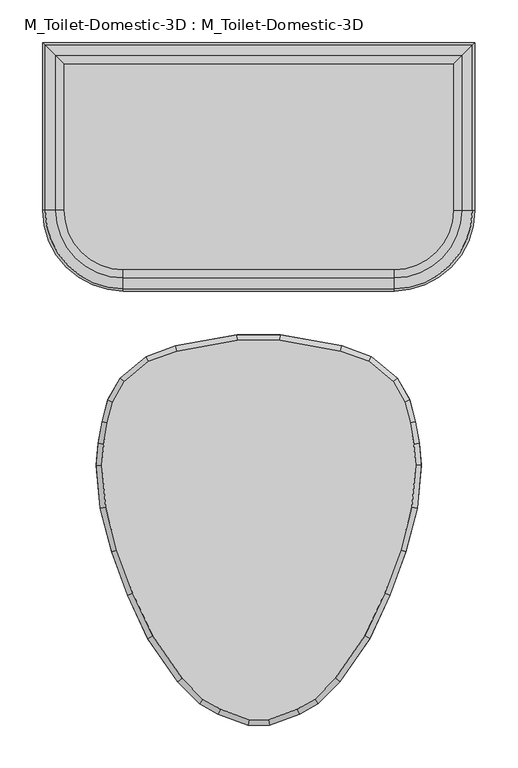
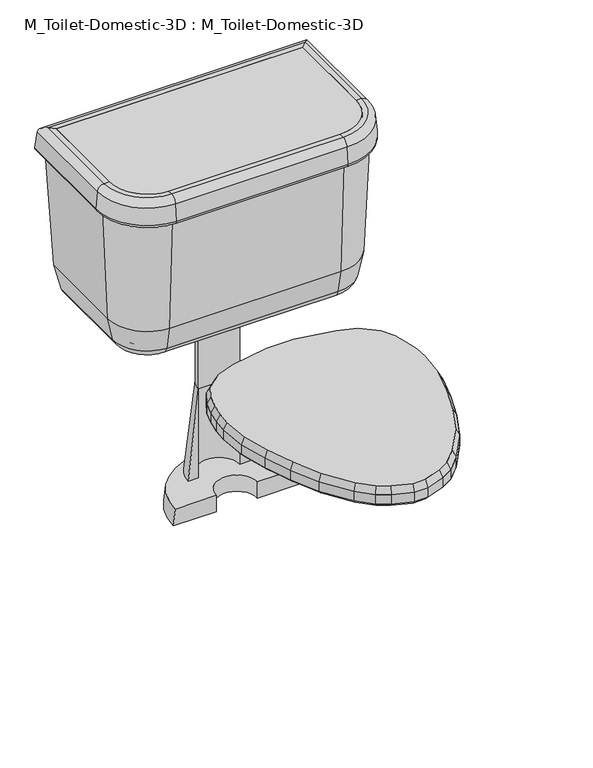
"""IFC4 building model written with IfcOpenShell, lengths in millimetres: flow terminal geometry, M_Toilet-Domestic-3D : M_Toilet-Domestic-3D."""

from ifc_helpers import new_model, si_unit, point, frame, frame_2d, origin, place, context, project, spatial, polyline, circle_curve, ellipse_curve, trimmed, segment, composite_curve, outline, extrude, faceted_brep, source, transform, mapped, element, save
from ifc_brep_helpers import plane_surface, cylinder_surface, revolved_surface, advanced_brep


def m_toilet_domestic_3d_m_toilet_domestic_3d_1a010dbe(model_context):
    return source(origin(), model_context, "Body", "SolidModel", [
        advanced_brep(
        [(177.8, 419.1, 387.2181453), (177.8, 419.1, 374.65), (177.8, 298.45, 374.65), (177.8, 298.45, 387.2181453), (192.8020829, 434.1020829, 387.2181453), (192.8020829, 298.45, 387.2181453), (211.4650931, 452.7650931, 402.4478636), (211.4650931, 298.45, 402.4478636), (218.7732506, 460.0732506, 438.15), (218.7732506, 298.45, 438.15), (228.5868869, 469.8868869, 654.05), (228.5868869, 298.45, 654.05), (228.5868869, 469.8868869, 704.85), (228.5868869, 298.45, 704.85), (237.91817, 479.21817, 704.85), (237.91817, 298.45, 704.85), (250.5698426, 491.8698426, 693.2568779), (250.5698426, 298.45, 693.2568779), (253.3960274, 494.6960274, 660.953439), (253.3960274, 298.45, 660.953439), (247.070191, 488.370191, 654.05), (247.070191, 298.45, 654.05), (241.3, 482.6, 654.05), (241.3, 298.45, 654.05), (231.4863636, 472.7863636, 438.15), (231.4863636, 298.45, 438.15), (222.3416824, 463.6416824, 393.4759963), (222.3416824, 298.45, 393.4759963), (197.8071664, 439.1071664, 374.65), (197.8071664, 298.45, 374.65), (158.75, 279.4, 387.2181453), (158.75, 279.4, 374.65), (158.75, 264.3979171, 387.2181453), (158.75, 245.7349069, 402.4478636), (158.75, 238.4267494, 438.15), (158.75, 228.6131131, 654.05), (158.75, 228.6131131, 704.85), (158.75, 219.28183, 704.85), (158.75, 206.6301574, 693.2568779), (158.75, 203.8039726, 660.953439), (158.75, 210.129809, 654.05), (158.75, 215.9, 654.05), (158.75, 225.7136364, 438.15), (158.75, 234.8583176, 393.4759963), (158.75, 259.3928336, 374.65), (-158.75, 279.4, 374.65), (-158.75, 279.4, 387.2181453), (-158.75, 264.3979171, 387.2181453), (-158.75, 245.7349069, 402.4478636), (-158.75, 238.4267494, 438.15), (-158.75, 228.6131131, 654.05), (-158.75, 228.6131131, 704.85), (-158.75, 219.28183, 704.85), (-158.75, 206.6301574, 693.2568779), (-158.75, 203.8039726, 660.953439), (-158.75, 210.129809, 654.05), (-158.75, 215.9, 654.05), (-158.75, 225.7136364, 438.15), (-158.75, 234.8583176, 393.4759963), (-158.75, 259.3928336, 374.65), (-177.8, 298.45, 387.2181453), (-177.8, 298.45, 374.65), (-192.8020829, 298.45, 387.2181453), (-211.4650931, 298.45, 402.4478636), (-218.7732506, 298.45, 438.15), (-228.5868869, 298.45, 654.05), (-228.5868869, 298.45, 704.85), (-237.91817, 298.45, 704.85), (-250.5698426, 298.45, 693.2568779), (-253.3960274, 298.45, 660.953439), (-247.070191, 298.45, 654.05), (-241.3, 298.45, 654.05), (-231.4863636, 298.45, 438.15), (-222.3416824, 298.45, 393.4759963), (-197.8071664, 298.45, 374.65), (-177.8, 419.1, 374.65), (-177.8, 419.1, 387.2181453), (-192.8020829, 434.1020829, 387.2181453), (-211.4650931, 452.7650931, 402.4478636), (-218.7732506, 460.0732506, 438.15), (-228.5868869, 469.8868869, 654.05), (-228.5868869, 469.8868869, 704.85), (-237.91817, 479.21817, 704.85), (-250.5698426, 491.8698426, 693.2568779), (-253.3960274, 494.6960274, 660.953439), (-247.070191, 488.370191, 654.05), (-241.3, 482.6, 654.05), (-231.4863636, 472.7863636, 438.15), (-222.3416824, 463.6416824, 393.4759963), (-197.8071664, 439.1071664, 374.65)],
        [
            (0, 1),
            (1, 2),
            (2, 3),
            (3, 0),
            (4, 0),
            (3, 5),
            (5, 4),
            (6, 4, ellipse_curve(frame((192.8020829, 434.1020829, 406.2681453), z_axis=(-0.7071067811865451, 0.7071067811865498, 0.0), x_axis=(-0.7071067811865497, -0.7071067811865452, 0.0)), 26.9407684, 19.05)),
            (5, 7, circle_curve(frame((192.8020829, 298.45, 406.2681453), z_axis=(0.0, -1.0, 0.0), x_axis=(1.0, 0.0, 0.0)), 19.05)),
            (7, 6),
            (8, 6),
            (7, 9),
            (9, 8),
            (10, 8),
            (9, 11),
            (11, 10),
            (12, 10),
            (11, 13),
            (13, 12),
            (14, 12),
            (13, 15),
            (15, 14),
            (16, 14, ellipse_curve(frame((237.91817, 479.21817, 692.15), z_axis=(0.7071067811865451, -0.7071067811865498, 0.0), x_axis=(0.7071067811865497, 0.7071067811865452, 0.0)), 17.9605122, 12.7)),
            (15, 17, circle_curve(frame((237.91817, 298.45, 692.15), z_axis=(0.0, 1.0, 0.0), x_axis=(1.0, 0.0, 0.0)), 12.7)),
            (17, 16),
            (18, 16),
            (17, 19),
            (19, 18),
            (20, 18, ellipse_curve(frame((247.070191, 488.370191, 660.4), z_axis=(0.7071067811865451, -0.7071067811865498, 0.0), x_axis=(0.7071067811865497, 0.7071067811865452, 0.0)), 8.9802561, 6.35)),
            (19, 21, circle_curve(frame((247.070191, 298.45, 660.4), z_axis=(0.0, 1.0, 0.0), x_axis=(1.0, 0.0, 0.0)), 6.35)),
            (21, 20),
            (22, 20),
            (21, 23),
            (23, 22),
            (24, 22),
            (23, 25),
            (25, 24),
            (26, 24),
            (25, 27),
            (27, 26),
            (28, 26, ellipse_curve(frame((197.8071664, 439.1071664, 400.05), z_axis=(0.7071067811865451, -0.7071067811865498, 0.0), x_axis=(0.7071067811865497, 0.7071067811865452, 0.0)), 35.9210245, 25.4)),
            (27, 29, circle_curve(frame((197.8071664, 298.45, 400.05), z_axis=(0.0, 1.0, 0.0), x_axis=(1.0, 0.0, 0.0)), 25.4)),
            (29, 28),
            (1, 28),
            (29, 2),
            (30, 3, circle_curve(frame((158.75, 298.45, 387.2181453), z_axis=(0.0, 0.0, 1.0), x_axis=(1.0, 0.0, 0.0)), 19.05)),
            (2, 31, circle_curve(frame((158.75, 298.45, 374.65), z_axis=(0.0, 0.0, -1.0), x_axis=(1.0, 0.0, 0.0)), 19.05)),
            (31, 30),
            (32, 5, circle_curve(frame((158.75, 298.45, 387.2181453), z_axis=(0.0, 0.0, 1.0), x_axis=(1.0, 0.0, 0.0)), 34.0520829)),
            (30, 32),
            (33, 7, circle_curve(frame((158.75, 298.45, 402.4478636), z_axis=(0.0, 0.0, 1.0), x_axis=(1.0, 0.0, 0.0)), 52.7150931)),
            (32, 33, circle_curve(frame((158.75, 264.3979171, 406.2681453), z_axis=(-1.0, 0.0, 0.0), x_axis=(0.0, -1.0, 0.0)), 19.05)),
            (34, 9, circle_curve(frame((158.75, 298.45, 438.15), z_axis=(0.0, 0.0, 1.0), x_axis=(1.0, 0.0, 0.0)), 60.0232506)),
            (33, 34),
            (35, 11, circle_curve(frame((158.75, 298.45, 654.05), z_axis=(0.0, 0.0, 1.0), x_axis=(1.0, 0.0, 0.0)), 69.8368869)),
            (34, 35),
            (36, 13, circle_curve(frame((158.75, 298.45, 704.85), z_axis=(0.0, 0.0, 1.0), x_axis=(1.0, 0.0, 0.0)), 69.8368869)),
            (35, 36),
            (37, 15, circle_curve(frame((158.75, 298.45, 704.85), z_axis=(0.0, 0.0, 1.0), x_axis=(1.0, 0.0, 0.0)), 79.16817)),
            (36, 37),
            (38, 17, circle_curve(frame((158.75, 298.45, 693.2568779), z_axis=(0.0, 0.0, 1.0), x_axis=(1.0, 0.0, 0.0)), 91.8198426)),
            (37, 38, circle_curve(frame((158.75, 219.28183, 692.15), z_axis=(1.0, 0.0, 0.0), x_axis=(0.0, -1.0, 0.0)), 12.7)),
            (39, 19, circle_curve(frame((158.75, 298.45, 660.953439), z_axis=(0.0, 0.0, 1.0), x_axis=(1.0, 0.0, 0.0)), 94.6460274)),
            (38, 39),
            (40, 21, circle_curve(frame((158.75, 298.45, 654.05), z_axis=(0.0, 0.0, 1.0), x_axis=(1.0, 0.0, 0.0)), 88.320191)),
            (39, 40, circle_curve(frame((158.75, 210.129809, 660.4), z_axis=(1.0, 0.0, 0.0), x_axis=(0.0, -1.0, 0.0)), 6.35)),
            (41, 23, circle_curve(frame((158.75, 298.45, 654.05), z_axis=(0.0, 0.0, 1.0), x_axis=(1.0, 0.0, 0.0)), 82.55)),
            (40, 41),
            (42, 25, circle_curve(frame((158.75, 298.45, 438.15), z_axis=(0.0, 0.0, 1.0), x_axis=(1.0, 0.0, 0.0)), 72.7363636)),
            (41, 42),
            (43, 27, circle_curve(frame((158.75, 298.45, 393.4759963), z_axis=(0.0, 0.0, 1.0), x_axis=(1.0, 0.0, 0.0)), 63.5916824)),
            (42, 43),
            (44, 29, circle_curve(frame((158.75, 298.45, 374.65), z_axis=(0.0, 0.0, 1.0), x_axis=(1.0, 0.0, 0.0)), 39.0571664)),
            (43, 44, circle_curve(frame((158.75, 259.3928336, 400.05), z_axis=(1.0, 0.0, 0.0), x_axis=(0.0, -1.0, 0.0)), 25.4)),
            (44, 31),
            (31, 45),
            (45, 46),
            (46, 30),
            (46, 47),
            (47, 32),
            (47, 48, circle_curve(frame((-158.75, 264.3979171, 406.2681453), z_axis=(-1.0, 0.0, 0.0), x_axis=(0.0, -1.0, 0.0)), 19.05)),
            (48, 33),
            (48, 49),
            (49, 34),
            (49, 50),
            (50, 35),
            (50, 51),
            (51, 36),
            (51, 52),
            (52, 37),
            (52, 53, circle_curve(frame((-158.75, 219.28183, 692.15), z_axis=(1.0, 0.0, 0.0), x_axis=(0.0, -1.0, 0.0)), 12.7)),
            (53, 38),
            (53, 54),
            (54, 39),
            (54, 55, circle_curve(frame((-158.75, 210.129809, 660.4), z_axis=(1.0, 0.0, 0.0), x_axis=(0.0, -1.0, 0.0)), 6.35)),
            (55, 40),
            (55, 56),
            (56, 41),
            (56, 57),
            (57, 42),
            (57, 58),
            (58, 43),
            (58, 59, circle_curve(frame((-158.75, 259.3928336, 400.05), z_axis=(1.0, 0.0, 0.0), x_axis=(0.0, -1.0, 0.0)), 25.4)),
            (59, 44),
            (59, 45),
            (60, 46, circle_curve(frame((-158.75, 298.45, 387.2181453), z_axis=(0.0, 0.0, 1.0), x_axis=(0.0, -1.0, 0.0)), 19.05)),
            (45, 61, circle_curve(frame((-158.75, 298.45, 374.65), z_axis=(0.0, 0.0, -1.0), x_axis=(0.0, -1.0, 0.0)), 19.05)),
            (61, 60),
            (62, 47, circle_curve(frame((-158.75, 298.45, 387.2181453), z_axis=(0.0, 0.0, 1.0), x_axis=(0.0, -1.0, 0.0)), 34.0520829)),
            (60, 62),
            (63, 48, circle_curve(frame((-158.75, 298.45, 402.4478636), z_axis=(0.0, 0.0, 1.0), x_axis=(0.0, -1.0, 0.0)), 52.7150931)),
            (62, 63, circle_curve(frame((-192.8020829, 298.45, 406.2681453), z_axis=(0.0, 1.0, 0.0), x_axis=(-1.0, 0.0, 0.0)), 19.05)),
            (64, 49, circle_curve(frame((-158.75, 298.45, 438.15), z_axis=(0.0, 0.0, 1.0), x_axis=(0.0, -1.0, 0.0)), 60.0232506)),
            (63, 64),
            (65, 50, circle_curve(frame((-158.75, 298.45, 654.05), z_axis=(0.0, 0.0, 1.0), x_axis=(0.0, -1.0, 0.0)), 69.8368869)),
            (64, 65),
            (66, 51, circle_curve(frame((-158.75, 298.45, 704.85), z_axis=(0.0, 0.0, 1.0), x_axis=(0.0, -1.0, 0.0)), 69.8368869)),
            (65, 66),
            (67, 52, circle_curve(frame((-158.75, 298.45, 704.85), z_axis=(0.0, 0.0, 1.0), x_axis=(0.0, -1.0, 0.0)), 79.16817)),
            (66, 67),
            (68, 53, circle_curve(frame((-158.75, 298.45, 693.2568779), z_axis=(0.0, 0.0, 1.0), x_axis=(0.0, -1.0, 0.0)), 91.8198426)),
            (67, 68, circle_curve(frame((-237.91817, 298.45, 692.15), z_axis=(0.0, -1.0, 0.0), x_axis=(-1.0, 0.0, 0.0)), 12.7)),
            (69, 54, circle_curve(frame((-158.75, 298.45, 660.953439), z_axis=(0.0, 0.0, 1.0), x_axis=(0.0, -1.0, 0.0)), 94.6460274)),
            (68, 69),
            (70, 55, circle_curve(frame((-158.75, 298.45, 654.05), z_axis=(0.0, 0.0, 1.0), x_axis=(0.0, -1.0, 0.0)), 88.320191)),
            (69, 70, circle_curve(frame((-247.070191, 298.45, 660.4), z_axis=(0.0, -1.0, 0.0), x_axis=(-1.0, 0.0, 0.0)), 6.35)),
            (71, 56, circle_curve(frame((-158.75, 298.45, 654.05), z_axis=(0.0, 0.0, 1.0), x_axis=(0.0, -1.0, 0.0)), 82.55)),
            (70, 71),
            (72, 57, circle_curve(frame((-158.75, 298.45, 438.15), z_axis=(0.0, 0.0, 1.0), x_axis=(0.0, -1.0, 0.0)), 72.7363636)),
            (71, 72),
            (73, 58, circle_curve(frame((-158.75, 298.45, 393.4759963), z_axis=(0.0, 0.0, 1.0), x_axis=(0.0, -1.0, 0.0)), 63.5916824)),
            (72, 73),
            (74, 59, circle_curve(frame((-158.75, 298.45, 374.65), z_axis=(0.0, 0.0, 1.0), x_axis=(0.0, -1.0, 0.0)), 39.0571664)),
            (73, 74, circle_curve(frame((-197.8071664, 298.45, 400.05), z_axis=(0.0, -1.0, 0.0), x_axis=(-1.0, 0.0, 0.0)), 25.4)),
            (74, 61),
            (61, 75),
            (75, 76),
            (76, 60),
            (76, 77),
            (77, 62),
            (77, 78, ellipse_curve(frame((-192.8020829, 434.1020829, 406.2681453), z_axis=(0.7071067811865498, 0.7071067811865451, 0.0), x_axis=(-0.7071067811865451, 0.70710678118655, 0.0)), 26.9407684, 19.05)),
            (78, 63),
            (78, 79),
            (79, 64),
            (79, 80),
            (80, 65),
            (80, 81),
            (81, 66),
            (81, 82),
            (82, 67),
            (82, 83, ellipse_curve(frame((-237.91817, 479.21817, 692.15), z_axis=(-0.7071067811865498, -0.7071067811865451, 0.0), x_axis=(0.7071067811865451, -0.70710678118655, 0.0)), 17.9605122, 12.7)),
            (83, 68),
            (83, 84),
            (84, 69),
            (84, 85, ellipse_curve(frame((-247.070191, 488.370191, 660.4), z_axis=(-0.7071067811865498, -0.7071067811865451, 0.0), x_axis=(0.7071067811865451, -0.70710678118655, 0.0)), 8.9802561, 6.35)),
            (85, 70),
            (85, 86),
            (86, 71),
            (86, 87),
            (87, 72),
            (87, 88),
            (88, 73),
            (88, 89, ellipse_curve(frame((-197.8071664, 439.1071664, 400.05), z_axis=(-0.7071067811865498, -0.7071067811865451, 0.0), x_axis=(0.7071067811865451, -0.70710678118655, 0.0)), 35.9210245, 25.4)),
            (89, 74),
            (89, 75),
            (75, 1),
            (0, 76),
            (4, 77),
            (6, 78),
            (8, 79),
            (10, 80),
            (12, 81),
            (14, 82),
            (16, 83),
            (18, 84),
            (20, 85),
            (22, 86),
            (24, 87),
            (26, 88),
            (28, 89),
        ],
        [
            plane_surface(frame((177.8, 419.1, 374.65), z_axis=(-1.0, 0.0, 0.0), x_axis=(0.0, -1.0, 0.0))),
            plane_surface(frame((177.8, 419.1, 387.2181453), z_axis=(0.0, 0.0, 1.0), x_axis=(0.0, -1.0, 0.0))),
            revolved_surface(polyline([(211.8520829, 298.45, 406.2681453), (211.8520829, 453.1520829260162, 406.2681453)]), (192.8020829, 419.1, 406.2681453), (0.0, -1.0, 0.0)),
            plane_surface(frame((211.4650931, 452.7650931, 402.4478636), z_axis=(-0.9796855721787505, 0.0, 0.2005397209153197), x_axis=(0.0, -1.0, 0.0))),
            plane_surface(frame((218.7732506, 460.0732506, 438.15), z_axis=(-0.9989685402102993, 0.0, 0.04540766091865541), x_axis=(0.0, -1.0, 0.0))),
            plane_surface(frame((228.5868869, 469.8868869, 654.05), z_axis=(-1.0, 0.0, 0.0), x_axis=(0.0, -1.0, 0.0))),
            plane_surface(frame((228.5868869, 469.8868869, 704.85), z_axis=(0.0, 0.0, 1.0), x_axis=(0.0, -1.0, 0.0))),
            cylinder_surface(frame((237.91817, 419.1, 692.15), z_axis=(0.0, 1.0, 0.0), x_axis=(1.0, 0.0, 0.0)), 12.7),
            plane_surface(frame((250.5698426, 491.8698426, 693.2568779), z_axis=(0.9961946980917448, 0.0, 0.08715574274766702), x_axis=(0.0, -1.0, 0.0))),
            cylinder_surface(frame((247.070191, 419.1, 660.4), z_axis=(0.0, 1.0, 0.0), x_axis=(1.0, 0.0, 0.0)), 6.35),
            plane_surface(frame((247.070191, 488.370191, 654.05), z_axis=(0.0, 0.0, -1.0), x_axis=(0.0, -1.0, 0.0))),
            plane_surface(frame((241.3, 482.6, 654.05), z_axis=(0.9989685402102995, 0.0, -0.04540766091865437), x_axis=(0.0, -1.0, 0.0))),
            plane_surface(frame((231.4863636, 472.7863636, 438.15), z_axis=(0.9796855721787479, 0.0, -0.2005397209153326), x_axis=(0.0, -1.0, 0.0))),
            cylinder_surface(frame((197.8071664, 419.1, 400.05), z_axis=(0.0, 1.0, 0.0), x_axis=(1.0, 0.0, 0.0)), 25.4),
            plane_surface(frame((197.8071664, 439.1071664, 374.65), z_axis=(0.0, 0.0, -1.0), x_axis=(0.0, -1.0, 0.0))),
            revolved_surface(polyline([(177.8, 298.45, 374.65), (177.8, 298.45, 387.2181453)]), (158.75, 298.45, 0.0), (0.0, 0.0, -1.0)),
            plane_surface(frame((158.75, 298.45, 387.2181453), z_axis=(0.0, 0.0, 1.0), x_axis=(1.0, 0.0, 0.0))),
            revolved_surface(trimmed(ellipse_curve(frame((192.8020829, 298.45, 406.2681453), z_axis=(0.0, -1.0, 0.0), x_axis=(1.0, 0.0, 0.0)), 19.05, 19.05), [point((192.8020829, 298.45, 387.2181453))], [point((211.4650931, 298.45, 402.4478636))], True, "CARTESIAN"), (158.75, 298.45, 0.0), (0.0, 0.0, -1.0)),
            revolved_surface(polyline([(211.4650931, 298.45, 402.4478636), (218.7732506, 298.45, 438.15)]), (158.75, 298.45, 0.0), (0.0, 0.0, -1.0)),
            revolved_surface(polyline([(218.7732506, 298.45, 438.15), (228.5868869, 298.45, 654.05)]), (158.75, 298.45, 0.0), (0.0, 0.0, -1.0)),
            revolved_surface(polyline([(228.5868869, 298.45, 654.05), (228.5868869, 298.45, 704.85)]), (158.75, 298.45, 0.0), (0.0, 0.0, -1.0)),
            plane_surface(frame((158.75, 298.45, 704.85), z_axis=(0.0, 0.0, 1.0), x_axis=(1.0, 0.0, 0.0))),
            revolved_surface(trimmed(ellipse_curve(frame((237.91817, 298.45, 692.15), z_axis=(0.0, 1.0, 0.0), x_axis=(1.0, 0.0, 0.0)), 12.7, 12.7), [point((237.91817, 298.45, 704.85))], [point((250.5698426, 298.45, 693.2568779))], True, "CARTESIAN"), (158.75, 298.45, 0.0), (0.0, 0.0, -1.0)),
            revolved_surface(polyline([(250.5698426, 298.45, 693.2568779), (253.3960274, 298.45, 660.953439)]), (158.75, 298.45, 0.0), (0.0, 0.0, -1.0)),
            revolved_surface(trimmed(ellipse_curve(frame((247.070191, 298.45, 660.4), z_axis=(0.0, 1.0, 0.0), x_axis=(1.0, 0.0, 0.0)), 6.35, 6.35), [point((253.3960274, 298.45, 660.953439))], [point((247.070191, 298.45, 654.05))], True, "CARTESIAN"), (158.75, 298.45, 0.0), (0.0, 0.0, -1.0)),
            plane_surface(frame((158.75, 298.45, 654.05), z_axis=(0.0, 0.0, -1.0), x_axis=(1.0, 0.0, 0.0))),
            revolved_surface(polyline([(241.3, 298.45, 654.05), (231.4863636, 298.45, 438.15)]), (158.75, 298.45, 0.0), (0.0, 0.0, -1.0)),
            revolved_surface(polyline([(231.4863636, 298.45, 438.15), (222.3416824, 298.45, 393.4759963)]), (158.75, 298.45, 0.0), (0.0, 0.0, -1.0)),
            revolved_surface(trimmed(ellipse_curve(frame((197.8071664, 298.45, 400.05), z_axis=(0.0, 1.0, 0.0), x_axis=(1.0, 0.0, 0.0)), 25.4, 25.4), [point((222.3416824, 298.45, 393.4759963))], [point((197.8071664, 298.45, 374.65))], True, "CARTESIAN"), (158.75, 298.45, 0.0), (0.0, 0.0, -1.0)),
            plane_surface(frame((158.75, 298.45, 374.65), z_axis=(0.0, 0.0, -1.0), x_axis=(1.0, 0.0, 0.0))),
            plane_surface(frame((158.75, 279.4, 374.65), z_axis=(0.0, 1.0, 0.0), x_axis=(-1.0, 0.0, 0.0))),
            plane_surface(frame((158.75, 279.4, 387.2181453), z_axis=(0.0, 0.0, 1.0), x_axis=(-1.0, 0.0, 0.0))),
            revolved_surface(polyline([(-158.75, 245.34791709999996, 406.2681453), (158.75, 245.34791709999996, 406.2681453)]), (158.75, 264.3979171, 406.2681453), (-1.0, 0.0, 0.0)),
            plane_surface(frame((158.75, 245.7349069, 402.4478636), z_axis=(0.0, 0.9796855721787505, 0.2005397209153197), x_axis=(-1.0, 0.0, 0.0))),
            plane_surface(frame((158.75, 238.4267494, 438.15), z_axis=(0.0, 0.9989685402102993, 0.04540766091865541), x_axis=(-1.0, 0.0, 0.0))),
            plane_surface(frame((158.75, 228.6131131, 654.05), z_axis=(0.0, 1.0, 0.0), x_axis=(-1.0, 0.0, 0.0))),
            plane_surface(frame((158.75, 228.6131131, 704.85), z_axis=(0.0, 0.0, 1.0), x_axis=(-1.0, 0.0, 0.0))),
            cylinder_surface(frame((158.75, 219.28183, 692.15), z_axis=(1.0, 0.0, 0.0), x_axis=(0.0, -1.0, 0.0)), 12.7),
            plane_surface(frame((158.75, 206.6301574, 693.2568779), z_axis=(0.0, -0.9961946980917448, 0.08715574274766702), x_axis=(-1.0, 0.0, 0.0))),
            cylinder_surface(frame((158.75, 210.129809, 660.4), z_axis=(1.0, 0.0, 0.0), x_axis=(0.0, -1.0, 0.0)), 6.35),
            plane_surface(frame((158.75, 210.129809, 654.05), z_axis=(0.0, 0.0, -1.0), x_axis=(-1.0, 0.0, 0.0))),
            plane_surface(frame((158.75, 215.9, 654.05), z_axis=(0.0, -0.9989685402102995, -0.04540766091865437), x_axis=(-1.0, 0.0, 0.0))),
            plane_surface(frame((158.75, 225.7136364, 438.15), z_axis=(0.0, -0.9796855721787479, -0.2005397209153326), x_axis=(-1.0, 0.0, 0.0))),
            cylinder_surface(frame((158.75, 259.3928336, 400.05), z_axis=(1.0, 0.0, 0.0), x_axis=(0.0, -1.0, 0.0)), 25.4),
            plane_surface(frame((158.75, 259.3928336, 374.65), z_axis=(0.0, 0.0, -1.0), x_axis=(-1.0, 0.0, 0.0))),
            revolved_surface(polyline([(-158.75, 279.4, 374.65), (-158.75, 279.4, 387.2181453)]), (-158.75, 298.45, 0.0), (0.0, 0.0, -1.0)),
            plane_surface(frame((-158.75, 298.45, 387.2181453), z_axis=(0.0, 0.0, 1.0), x_axis=(0.0, -1.0, 0.0))),
            revolved_surface(trimmed(ellipse_curve(frame((-158.75, 264.3979171, 406.2681453), z_axis=(-1.0, 0.0, 0.0), x_axis=(0.0, -1.0, 0.0)), 19.05, 19.05), [point((-158.75, 264.3979171, 387.2181453))], [point((-158.75, 245.7349069, 402.4478636))], True, "CARTESIAN"), (-158.75, 298.45, 0.0), (0.0, 0.0, -1.0)),
            revolved_surface(polyline([(-158.75, 245.7349069, 402.4478636), (-158.75, 238.4267494, 438.15)]), (-158.75, 298.45, 0.0), (0.0, 0.0, -1.0)),
            revolved_surface(polyline([(-158.75, 238.4267494, 438.15), (-158.75, 228.6131131, 654.05)]), (-158.75, 298.45, 0.0), (0.0, 0.0, -1.0)),
            revolved_surface(polyline([(-158.75, 228.6131131, 654.05), (-158.75, 228.6131131, 704.85)]), (-158.75, 298.45, 0.0), (0.0, 0.0, -1.0)),
            plane_surface(frame((-158.75, 298.45, 704.85), z_axis=(0.0, 0.0, 1.0), x_axis=(0.0, -1.0, 0.0))),
            revolved_surface(trimmed(ellipse_curve(frame((-158.75, 219.28183, 692.15), z_axis=(1.0, 0.0, 0.0), x_axis=(0.0, -1.0, 0.0)), 12.7, 12.7), [point((-158.75, 219.28183, 704.85))], [point((-158.75, 206.6301574, 693.2568779))], True, "CARTESIAN"), (-158.75, 298.45, 0.0), (0.0, 0.0, -1.0)),
            revolved_surface(polyline([(-158.75, 206.6301574, 693.2568779), (-158.75, 203.8039726, 660.953439)]), (-158.75, 298.45, 0.0), (0.0, 0.0, -1.0)),
            revolved_surface(trimmed(ellipse_curve(frame((-158.75, 210.129809, 660.4), z_axis=(1.0, 0.0, 0.0), x_axis=(0.0, -1.0, 0.0)), 6.35, 6.35), [point((-158.75, 203.8039726, 660.953439))], [point((-158.75, 210.129809, 654.05))], True, "CARTESIAN"), (-158.75, 298.45, 0.0), (0.0, 0.0, -1.0)),
            plane_surface(frame((-158.75, 298.45, 654.05), z_axis=(0.0, 0.0, -1.0), x_axis=(0.0, -1.0, 0.0))),
            revolved_surface(polyline([(-158.75, 215.9, 654.05), (-158.75, 225.7136364, 438.15)]), (-158.75, 298.45, 0.0), (0.0, 0.0, -1.0)),
            revolved_surface(polyline([(-158.75, 225.7136364, 438.15), (-158.75, 234.8583176, 393.4759963)]), (-158.75, 298.45, 0.0), (0.0, 0.0, -1.0)),
            revolved_surface(trimmed(ellipse_curve(frame((-158.75, 259.3928336, 400.05), z_axis=(1.0, 0.0, 0.0), x_axis=(0.0, -1.0, 0.0)), 25.4, 25.4), [point((-158.75, 234.8583176, 393.4759963))], [point((-158.75, 259.3928336, 374.65))], True, "CARTESIAN"), (-158.75, 298.45, 0.0), (0.0, 0.0, -1.0)),
            plane_surface(frame((-158.75, 298.45, 374.65), z_axis=(0.0, 0.0, -1.0), x_axis=(0.0, -1.0, 0.0))),
            plane_surface(frame((-177.8, 298.45, 374.65), z_axis=(1.0, 0.0, 0.0), x_axis=(0.0, 1.0, 0.0))),
            plane_surface(frame((-177.8, 298.45, 387.2181453), z_axis=(0.0, 0.0, 1.0), x_axis=(0.0, 1.0, 0.0))),
            revolved_surface(polyline([(-211.8520829, 453.15208292601636, 406.2681453), (-211.8520829, 298.45, 406.2681453)]), (-192.8020829, 298.45, 406.2681453), (0.0, 1.0, 0.0)),
            plane_surface(frame((-211.4650931, 298.45, 402.4478636), z_axis=(0.9796855721787505, 0.0, 0.2005397209153197), x_axis=(0.0, 1.0, 0.0))),
            plane_surface(frame((-218.7732506, 298.45, 438.15), z_axis=(0.9989685402102993, 0.0, 0.04540766091865541), x_axis=(0.0, 1.0, 0.0))),
            plane_surface(frame((-228.5868869, 298.45, 654.05), z_axis=(1.0, 0.0, 0.0), x_axis=(0.0, 1.0, 0.0))),
            plane_surface(frame((-228.5868869, 298.45, 704.85), z_axis=(0.0, 0.0, 1.0), x_axis=(0.0, 1.0, 0.0))),
            cylinder_surface(frame((-237.91817, 298.45, 692.15), z_axis=(0.0, -1.0, 0.0), x_axis=(-1.0, 0.0, 0.0)), 12.7),
            plane_surface(frame((-250.5698426, 298.45, 693.2568779), z_axis=(-0.9961946980917448, 0.0, 0.08715574274766702), x_axis=(0.0, 1.0, 0.0))),
            cylinder_surface(frame((-247.070191, 298.45, 660.4), z_axis=(0.0, -1.0, 0.0), x_axis=(-1.0, 0.0, 0.0)), 6.35),
            plane_surface(frame((-247.070191, 298.45, 654.05), z_axis=(0.0, 0.0, -1.0), x_axis=(0.0, 1.0, 0.0))),
            plane_surface(frame((-241.3, 298.45, 654.05), z_axis=(-0.9989685402102995, 0.0, -0.04540766091865437), x_axis=(0.0, 1.0, 0.0))),
            plane_surface(frame((-231.4863636, 298.45, 438.15), z_axis=(-0.9796855721787479, 0.0, -0.2005397209153326), x_axis=(0.0, 1.0, 0.0))),
            cylinder_surface(frame((-197.8071664, 298.45, 400.05), z_axis=(0.0, -1.0, 0.0), x_axis=(-1.0, 0.0, 0.0)), 25.4),
            plane_surface(frame((-197.8071664, 298.45, 374.65), z_axis=(0.0, 0.0, -1.0), x_axis=(0.0, 1.0, 0.0))),
            plane_surface(frame((-177.8, 419.1, 374.65), z_axis=(0.0, -1.0, 0.0), x_axis=(1.0, 0.0, 0.0))),
            plane_surface(frame((-177.8, 419.1, 387.2181453), z_axis=(0.0, 0.0, 1.0), x_axis=(1.0, 0.0, 0.0))),
            revolved_surface(polyline([(211.85208292601635, 453.15208290000004, 406.2681453), (-211.85208292601618, 453.15208290000004, 406.2681453)]), (-177.8, 434.1020829, 406.2681453), (1.0, 0.0, 0.0)),
            plane_surface(frame((-211.4650931, 452.7650931, 402.4478636), z_axis=(0.0, -0.9796855721787505, 0.2005397209153197), x_axis=(1.0, 0.0, 0.0))),
            plane_surface(frame((-218.7732506, 460.0732506, 438.15), z_axis=(0.0, -0.9989685402102993, 0.04540766091865541), x_axis=(1.0, 0.0, 0.0))),
            plane_surface(frame((-228.5868869, 469.8868869, 654.05), z_axis=(0.0, -1.0, 0.0), x_axis=(1.0, 0.0, 0.0))),
            plane_surface(frame((-228.5868869, 469.8868869, 704.85), z_axis=(0.0, 0.0, 1.0), x_axis=(1.0, 0.0, 0.0))),
            cylinder_surface(frame((-177.8, 479.21817, 692.15), z_axis=(-1.0, 0.0, 0.0), x_axis=(0.0, 1.0, 0.0)), 12.7),
            plane_surface(frame((-250.5698426, 491.8698426, 693.2568779), z_axis=(0.0, 0.9961946980917448, 0.08715574274766702), x_axis=(1.0, 0.0, 0.0))),
            cylinder_surface(frame((-177.8, 488.370191, 660.4), z_axis=(-1.0, 0.0, 0.0), x_axis=(0.0, 1.0, 0.0)), 6.35),
            plane_surface(frame((-247.070191, 488.370191, 654.05), z_axis=(0.0, 0.0, -1.0), x_axis=(1.0, 0.0, 0.0))),
            plane_surface(frame((-241.3, 482.6, 654.05), z_axis=(0.0, 0.9989685402102995, -0.04540766091865437), x_axis=(1.0, 0.0, 0.0))),
            plane_surface(frame((-231.4863636, 472.7863636, 438.15), z_axis=(0.0, 0.9796855721787479, -0.2005397209153326), x_axis=(1.0, 0.0, 0.0))),
            cylinder_surface(frame((-177.8, 439.1071664, 400.05), z_axis=(-1.0, 0.0, 0.0), x_axis=(0.0, 1.0, 0.0)), 25.4),
            plane_surface(frame((-197.8071664, 439.1071664, 374.65), z_axis=(0.0, 0.0, -1.0), x_axis=(1.0, 0.0, 0.0))),
        ],
        [
            (0, [[1, 2, 3, 4]]),
            (1, [[5, -4, 6, 7]]),
            (2, [[8, -7, 9, 10]]),
            (3, [[11, -10, 12, 13]]),
            (4, [[14, -13, 15, 16]]),
            (5, [[17, -16, 18, 19]]),
            (6, [[20, -19, 21, 22]]),
            (7, [[23, -22, 24, 25]]),
            (8, [[26, -25, 27, 28]]),
            (9, [[29, -28, 30, 31]]),
            (10, [[32, -31, 33, 34]]),
            (11, [[35, -34, 36, 37]]),
            (12, [[38, -37, 39, 40]]),
            (13, [[41, -40, 42, 43]]),
            (14, [[44, -43, 45, -2]]),
            (15, [[46, -3, 47, 48]]),
            (16, [[49, -6, -46, 50]]),
            (17, [[51, -9, -49, 52]]),
            (18, [[53, -12, -51, 54]]),
            (19, [[55, -15, -53, 56]]),
            (20, [[57, -18, -55, 58]]),
            (21, [[59, -21, -57, 60]]),
            (22, [[61, -24, -59, 62]]),
            (23, [[63, -27, -61, 64]]),
            (24, [[65, -30, -63, 66]]),
            (25, [[67, -33, -65, 68]]),
            (26, [[69, -36, -67, 70]]),
            (27, [[71, -39, -69, 72]]),
            (28, [[73, -42, -71, 74]]),
            (29, [[-47, -45, -73, 75]]),
            (30, [[-48, 76, 77, 78]]),
            (31, [[-50, -78, 79, 80]]),
            (32, [[-52, -80, 81, 82]]),
            (33, [[-54, -82, 83, 84]]),
            (34, [[-56, -84, 85, 86]]),
            (35, [[-58, -86, 87, 88]]),
            (36, [[-60, -88, 89, 90]]),
            (37, [[-62, -90, 91, 92]]),
            (38, [[-64, -92, 93, 94]]),
            (39, [[-66, -94, 95, 96]]),
            (40, [[-68, -96, 97, 98]]),
            (41, [[-70, -98, 99, 100]]),
            (42, [[-72, -100, 101, 102]]),
            (43, [[-74, -102, 103, 104]]),
            (44, [[-75, -104, 105, -76]]),
            (45, [[106, -77, 107, 108]]),
            (46, [[109, -79, -106, 110]]),
            (47, [[111, -81, -109, 112]]),
            (48, [[113, -83, -111, 114]]),
            (49, [[115, -85, -113, 116]]),
            (50, [[117, -87, -115, 118]]),
            (51, [[119, -89, -117, 120]]),
            (52, [[121, -91, -119, 122]]),
            (53, [[123, -93, -121, 124]]),
            (54, [[125, -95, -123, 126]]),
            (55, [[127, -97, -125, 128]]),
            (56, [[129, -99, -127, 130]]),
            (57, [[131, -101, -129, 132]]),
            (58, [[133, -103, -131, 134]]),
            (59, [[-107, -105, -133, 135]]),
            (60, [[-108, 136, 137, 138]]),
            (61, [[-110, -138, 139, 140]]),
            (62, [[-112, -140, 141, 142]]),
            (63, [[-114, -142, 143, 144]]),
            (64, [[-116, -144, 145, 146]]),
            (65, [[-118, -146, 147, 148]]),
            (66, [[-120, -148, 149, 150]]),
            (67, [[-122, -150, 151, 152]]),
            (68, [[-124, -152, 153, 154]]),
            (69, [[-126, -154, 155, 156]]),
            (70, [[-128, -156, 157, 158]]),
            (71, [[-130, -158, 159, 160]]),
            (72, [[-132, -160, 161, 162]]),
            (73, [[-134, -162, 163, 164]]),
            (74, [[-135, -164, 165, -136]]),
            (75, [[-137, 166, -1, 167]]),
            (76, [[-139, -167, -5, 168]]),
            (77, [[-141, -168, -8, 169]]),
            (78, [[-143, -169, -11, 170]]),
            (79, [[-145, -170, -14, 171]]),
            (80, [[-147, -171, -17, 172]]),
            (81, [[-149, -172, -20, 173]]),
            (82, [[-151, -173, -23, 174]]),
            (83, [[-153, -174, -26, 175]]),
            (84, [[-155, -175, -29, 176]]),
            (85, [[-157, -176, -32, 177]]),
            (86, [[-159, -177, -35, 178]]),
            (87, [[-161, -178, -38, 179]]),
            (88, [[-163, -179, -41, 180]]),
            (89, [[-165, -180, -44, -166]]),
        ],
    ),
        extrude(outline(composite_curve([segment(trimmed(circle_curve(frame_2d((0.0, 342.9)), 38.1), [point((-38.1, 342.9))], [point((38.1, 342.9))], False, "CARTESIAN"), True, "CONTINUOUS"), segment(polyline([(38.1, 342.9), (-38.1, 342.9)]), True, "CONTINUOUS")], self_intersect=False)), frame((0.0, 0.0, 206.375), z_axis=(0.0, 0.0, 1.0), x_axis=(1.0, 0.0, 0.0)), (0.0, 0.0, 1.0), 130.175),
        extrude(outline(composite_curve([segment(polyline([(228.5868869, 469.8868869), (228.5868869, 298.45)]), True, "CONTINUOUS"), segment(trimmed(circle_curve(frame_2d((158.75, 298.45)), 69.8368869), [point((228.5868869, 298.45))], [point((158.75, 228.6131131))], False, "CARTESIAN"), True, "CONTINUOUS"), segment(polyline([(158.75, 228.6131131), (-158.75, 228.6131131)]), True, "CONTINUOUS"), segment(trimmed(circle_curve(frame_2d((-158.75, 298.45)), 69.8368869), [point((-158.75, 228.6131131))], [point((-228.5868869, 298.45))], False, "CARTESIAN"), True, "CONTINUOUS"), segment(polyline([(-228.5868869, 298.45), (-228.5868869, 469.8868869), (228.5868869, 469.8868869)]), True, "CONTINUOUS")], self_intersect=False)), frame((0.0, 0.0, 654.05), z_axis=(0.0, 0.0, 1.0), x_axis=(1.0, 0.0, 0.0)), (0.0, 0.0, 1.0), 50.8),
        faceted_brep([(-157.6293435, 97.472128, 400.05), (-171.060664, 73.773864, 400.05), (-177.5851102, 49.4242991, 400.05), (-181.9845715, 24.4737144, 400.05), (-184.125744, 0.0, 400.05), (-179.7950716, -49.4998127, 400.05), (-166.347, -99.688699, 400.05), (-148.0469602, -149.9676451, 400.05), (-124.7045808, -200.0255393, 400.05), (-90.0971582, -249.9125941, 400.05), (-65.691017, -274.3187354, 400.05), (-44.8990862, -286.3229622, 400.05), (-11.5803237, -298.45, 400.05), (11.5803237, -298.45, 400.05), (44.8990862, -286.3229622, 400.05), (65.691017, -274.3187354, 400.05), (90.0971582, -249.9125941, 400.05), (124.7045808, -200.0255393, 400.05), (148.0469602, -149.9676451, 400.05), (166.347, -99.688699, 400.05), (179.7950716, -49.4998127, 400.05), (184.125744, 0.0, 400.05), (181.9845715, 24.4737144, 400.05), (177.5851102, 49.4242991, 400.05), (171.060664, 73.773864, 400.05), (157.6293435, 97.472128, 400.05), (129.0942628, 121.4159037, 400.05), (95.7755003, 133.5429415, 400.05), (24.844447, 146.05, 400.05), (-24.844447, 146.05, 400.05), (-95.7755003, 133.5429415, 400.05), (-129.0942628, 121.4159037, 400.05), (-162.5887836, 101.6, 387.2181453), (-132.3182423, 127.0, 387.2181453), (-97.4252791, 139.7, 387.2181453), (-25.4, 152.4, 387.2181453), (25.4, 152.4, 387.2181453), (97.4252791, 139.7, 387.2181453), (132.3182423, 127.0, 387.2181453), (162.5887836, 101.6, 387.2181453), (176.9845865, 76.2, 387.2181453), (183.790496, 50.8, 387.2181453), (188.2862441, 25.3033453, 387.2181453), (190.5, 0.0, 387.2181453), (186.0724883, -50.6066907, 387.2181453), (172.4088722, -101.6, 387.2181453), (153.9191843, -152.4, 387.2181453), (130.2307553, -203.2, 387.2181453), (94.9900085, -254.0, 387.2181453), (69.5900085, -279.4, 387.2181453), (47.5929632, -292.1, 387.2181453), (12.7, -304.8, 387.2181453), (-12.7, -304.8, 387.2181453), (-47.5929632, -292.1, 387.2181453), (-69.5900085, -279.4, 387.2181453), (-94.9900085, -254.0, 387.2181453), (-130.2307553, -203.2, 387.2181453), (-153.9191843, -152.4, 387.2181453), (-172.4088722, -101.6, 387.2181453), (-186.0724883, -50.6066907, 387.2181453), (-190.5, 0.0, 387.2181453), (-188.2862441, 25.3033453, 387.2181453), (-183.790496, 50.8, 387.2181453), (-176.9845865, 76.2, 387.2181453)], [[[0, 1, 2, 3, 4, 5, 6, 7, 8, 9, 10, 11, 12, 13, 14, 15, 16, 17, 18, 19, 20, 21, 22, 23, 24, 25, 26, 27, 28, 29, 30, 31]], [[32, 33, 34, 35, 36, 37, 38, 39, 40, 41, 42, 43, 44, 45, 46, 47, 48, 49, 50, 51, 52, 53, 54, 55, 56, 57, 58, 59, 60, 61, 62, 63]], [[32, 63, 1, 0]], [[63, 62, 2, 1]], [[62, 61, 3, 2]], [[61, 60, 4, 3]], [[60, 59, 5, 4]], [[59, 58, 6, 5]], [[58, 57, 7, 6]], [[57, 56, 8, 7]], [[56, 55, 9, 8]], [[55, 54, 10, 9]], [[54, 53, 11, 10]], [[53, 52, 12, 11]], [[52, 51, 13, 12]], [[51, 50, 14, 13]], [[50, 49, 15, 14]], [[49, 48, 16, 15]], [[48, 47, 17, 16]], [[47, 46, 18, 17]], [[46, 45, 19, 18]], [[45, 44, 20, 19]], [[44, 43, 21, 20]], [[43, 42, 22, 21]], [[42, 41, 23, 22]], [[41, 40, 24, 23]], [[40, 39, 25, 24]], [[39, 38, 26, 25]], [[38, 37, 27, 26]], [[37, 36, 28, 27]], [[36, 35, 29, 28]], [[35, 34, 30, 29]], [[34, 33, 31, 30]], [[33, 32, 0, 31]]]),
        advanced_brep(
        [(-38.1, 342.9, 206.375), (-57.15, 342.9, 31.75), (-38.1, 342.9, 31.75), (38.1, 342.9, 206.375), (38.1, 342.9, 31.75), (57.15, 342.9, 31.75)],
        [
            (0, 1),
            (1, 2),
            (2, 0),
            (3, 4),
            (4, 5),
            (5, 3),
            (5, 1, circle_curve(frame((0.0, 342.9, 31.75), z_axis=(0.0, 0.0, 1.0), x_axis=(-1.0, 0.0, 0.0)), 57.15)),
            (0, 3, circle_curve(frame((0.0, 342.9, 206.375), z_axis=(0.0, 0.0, -1.0), x_axis=(-1.0, 0.0, 0.0)), 38.1)),
            (4, 2, circle_curve(frame((0.0, 342.9, 31.75), z_axis=(0.0, 0.0, 1.0), x_axis=(-1.0, 0.0, 0.0)), 38.1)),
        ],
        [
            plane_surface(frame((0.0, 342.9, 31.75), z_axis=(0.0, -1.0, 0.0), x_axis=(-1.0, 0.0, 0.0))),
            plane_surface(frame((0.0, 342.9, 31.75), z_axis=(0.0, -1.0, 0.0), x_axis=(1.0, 0.0, 0.0))),
            revolved_surface(polyline([(-38.1, 342.9, 206.375), (-57.15, 342.9, 31.75)]), (0.0, 342.9, 31.75), (0.0, 0.0, -1.0)),
            plane_surface(frame((0.0, 342.9, 31.75), z_axis=(0.0, 0.0, -1.0), x_axis=(-1.0, 0.0, 0.0))),
            revolved_surface(polyline([(-38.1, 342.9, 31.75), (-38.1, 342.9, 206.375)]), (0.0, 342.9, 31.75), (0.0, 0.0, -1.0)),
        ],
        [
            (0, [[1, 2, 3]]),
            (1, [[4, 5, 6]]),
            (2, [[7, -1, 8, -6]]),
            (3, [[9, -2, -7, -5]]),
            (4, [[-8, -3, -9, -4]]),
        ],
    ),
        advanced_brep(
        [(-117.7636364, 285.75, 0.0), (-38.1, 285.75, 0.0), (-38.1, 285.75, 31.75), (-114.3, 285.75, 31.75), (117.7636364, 285.75, 0.0), (114.3, 285.75, 31.75), (38.1, 285.75, 31.75), (38.1, 285.75, 0.0)],
        [
            (0, 1),
            (1, 2),
            (2, 3),
            (3, 0),
            (4, 5),
            (5, 6),
            (6, 7),
            (7, 4),
            (7, 1, circle_curve(frame((0.0, 285.75, 0.0), z_axis=(0.0, 0.0, 1.0), x_axis=(-1.0, 0.0, 0.0)), 38.1)),
            (0, 4, circle_curve(frame((0.0, 285.75, 0.0), z_axis=(0.0, 0.0, -1.0), x_axis=(-1.0, 0.0, 0.0)), 117.7636364)),
            (6, 2, circle_curve(frame((0.0, 285.75, 31.75), z_axis=(0.0, 0.0, 1.0), x_axis=(-1.0, 0.0, 0.0)), 38.1)),
            (5, 3, circle_curve(frame((0.0, 285.75, 31.75), z_axis=(0.0, 0.0, 1.0), x_axis=(-1.0, 0.0, 0.0)), 114.3)),
        ],
        [
            plane_surface(frame((0.0, 285.75, -304.8), z_axis=(0.0, -1.0, 0.0), x_axis=(-1.0, 0.0, 0.0))),
            plane_surface(frame((0.0, 285.75, -304.8), z_axis=(0.0, -1.0, 0.0), x_axis=(1.0, 0.0, 0.0))),
            plane_surface(frame((0.0, 285.75, 0.0), z_axis=(0.0, 0.0, -1.0), x_axis=(-1.0, 0.0, 0.0))),
            revolved_surface(polyline([(-38.1, 285.75, 0.0), (-38.1, 285.75, 31.75)]), (0.0, 285.75, -304.8), (0.0, 0.0, -1.0)),
            plane_surface(frame((0.0, 285.75, 31.75), z_axis=(0.0, 0.0, 1.0), x_axis=(-1.0, 0.0, 0.0))),
            revolved_surface(polyline([(-114.3, 285.75, 31.75), (-117.7636364, 285.75, 0.0)]), (0.0, 285.75, -304.8), (0.0, 0.0, -1.0)),
        ],
        [
            (0, [[1, 2, 3, 4]]),
            (1, [[5, 6, 7, 8]]),
            (2, [[9, -1, 10, -8]]),
            (3, [[11, -2, -9, -7]]),
            (4, [[12, -3, -11, -6]]),
            (5, [[-10, -4, -12, -5]]),
        ],
    ),
        extrude(outline(composite_curve([segment(polyline([(177.8, 419.1), (177.8, 298.45)]), True, "CONTINUOUS"), segment(trimmed(circle_curve(frame_2d((158.75, 298.45)), 19.05), [point((177.8, 298.45))], [point((158.75, 279.4))], False, "CARTESIAN"), True, "CONTINUOUS"), segment(polyline([(158.75, 279.4), (-158.75, 279.4)]), True, "CONTINUOUS"), segment(trimmed(circle_curve(frame_2d((-158.75, 298.45)), 19.05), [point((-158.75, 279.4))], [point((-177.8, 298.45))], False, "CARTESIAN"), True, "CONTINUOUS"), segment(polyline([(-177.8, 298.45), (-177.8, 419.1), (177.8, 419.1)]), True, "CONTINUOUS")], self_intersect=False)), frame((0.0, 0.0, 374.65), z_axis=(0.0, 0.0, 1.0), x_axis=(1.0, 0.0, 0.0)), (0.0, 0.0, 1.0), 12.5681453),
        faceted_brep([(-97.4252791, 139.7, 368.3), (-132.3182423, 127.0, 368.3), (-162.5887836, 101.6, 368.3), (-176.9845865, 76.2, 368.3), (-183.790496, 50.8, 368.3), (-188.2862441, 25.3033453, 368.3), (-190.5, 0.0, 368.3), (-186.0724883, -50.6066907, 368.3), (-172.4088722, -101.6, 368.3), (-153.9191843, -152.4, 368.3), (-130.2307553, -203.2, 368.3), (-94.9900085, -254.0, 368.3), (-69.5900085, -279.4, 368.3), (-47.5929632, -292.1, 368.3), (-12.7, -304.8, 368.3), (12.7, -304.8, 368.3), (47.5929632, -292.1, 368.3), (69.5900085, -279.4, 368.3), (94.9900085, -254.0, 368.3), (130.2307553, -203.2, 368.3), (153.9191843, -152.4, 368.3), (172.4088722, -101.6, 368.3), (186.0724883, -50.6066907, 368.3), (190.5, 0.0, 368.3), (188.2862441, 25.3033453, 368.3), (183.790496, 50.8, 368.3), (176.9845865, 76.2, 368.3), (162.5887836, 101.6, 368.3), (132.3182423, 127.0, 368.3), (97.4252791, 139.7, 368.3), (25.4, 152.4, 368.3), (-25.4, 152.4, 368.3), (-95.7755003, 133.5429415, 361.95), (-24.844447, 146.05, 361.95), (24.844447, 146.05, 361.95), (95.7755003, 133.5429415, 361.95), (129.0942628, 121.4159037, 361.95), (157.6293435, 97.472128, 361.95), (171.060664, 73.773864, 361.95), (177.5851102, 49.4242991, 361.95), (181.9845715, 24.4737144, 361.95), (184.125744, 0.0, 361.95), (179.7950716, -49.4998127, 361.95), (166.347, -99.688699, 361.95), (148.0469602, -149.9676451, 361.95), (124.7045808, -200.0255393, 361.95), (90.0971582, -249.9125941, 361.95), (65.691017, -274.3187354, 361.95), (44.8990862, -286.3229622, 361.95), (11.5803237, -298.45, 361.95), (-11.5803237, -298.45, 361.95), (-44.8990862, -286.3229622, 361.95), (-65.691017, -274.3187354, 361.95), (-90.0971582, -249.9125941, 361.95), (-124.7045808, -200.0255393, 361.95), (-148.0469602, -149.9676451, 361.95), (-166.347, -99.688699, 361.95), (-179.7950716, -49.4998127, 361.95), (-184.125744, 0.0, 361.95), (-181.9845715, 24.4737144, 361.95), (-177.5851102, 49.4242991, 361.95), (-171.060664, 73.773864, 361.95), (-157.6293435, 97.472128, 361.95), (-129.0942628, 121.4159037, 361.95)], [[[0, 1, 2, 3, 4, 5, 6, 7, 8, 9, 10, 11, 12, 13, 14, 15, 16, 17, 18, 19, 20, 21, 22, 23, 24, 25, 26, 27, 28, 29, 30, 31]], [[32, 33, 34, 35, 36, 37, 38, 39, 40, 41, 42, 43, 44, 45, 46, 47, 48, 49, 50, 51, 52, 53, 54, 55, 56, 57, 58, 59, 60, 61, 62, 63]], [[32, 63, 1, 0]], [[63, 62, 2, 1]], [[62, 61, 3, 2]], [[61, 60, 4, 3]], [[60, 59, 5, 4]], [[59, 58, 6, 5]], [[58, 57, 7, 6]], [[57, 56, 8, 7]], [[56, 55, 9, 8]], [[55, 54, 10, 9]], [[54, 53, 11, 10]], [[53, 52, 12, 11]], [[52, 51, 13, 12]], [[51, 50, 14, 13]], [[50, 49, 15, 14]], [[49, 48, 16, 15]], [[48, 47, 17, 16]], [[47, 46, 18, 17]], [[46, 45, 19, 18]], [[45, 44, 20, 19]], [[44, 43, 21, 20]], [[43, 42, 22, 21]], [[42, 41, 23, 22]], [[41, 40, 24, 23]], [[40, 39, 25, 24]], [[39, 38, 26, 25]], [[38, 37, 27, 26]], [[37, 36, 28, 27]], [[36, 35, 29, 28]], [[35, 34, 30, 29]], [[34, 33, 31, 30]], [[33, 32, 0, 31]]]),
        extrude(outline(polyline([(-162.5887836, 101.6), (-132.3182423, 127.0), (-97.4252791, 139.7), (-25.4, 152.4), (25.4, 152.4), (97.4252791, 139.7), (132.3182423, 127.0), (162.5887836, 101.6), (176.9845865, 76.2), (183.790496, 50.8), (188.2862441, 25.3033453), (190.5, 0.0), (186.0724883, -50.6066907), (172.4088722, -101.6), (153.9191843, -152.4), (130.2307553, -203.2), (94.9900085, -254.0), (69.5900085, -279.4), (47.5929632, -292.1), (12.7, -304.8), (-12.7, -304.8), (-47.5929632, -292.1), (-69.5900085, -279.4), (-94.9900085, -254.0), (-130.2307553, -203.2), (-153.9191843, -152.4), (-172.4088722, -101.6), (-186.0724883, -50.6066907), (-190.5, 0.0), (-188.2862441, 25.3033453), (-183.790496, 50.8), (-176.9845865, 76.2), (-162.5887836, 101.6)])), frame((0.0, 0.0, 368.3), z_axis=(0.0, 0.0, 1.0), x_axis=(1.0, 0.0, 0.0)), (0.0, 0.0, 1.0), 19.05),
    ])


if __name__ == "__main__":
    model = new_model("IFC4")
    model_context = context("Model", 3, world=origin())
    ifc_project = project(units=[si_unit("LENGTHUNIT", "METRE", prefix="MILLI")], contexts=[model_context])
    site = spatial("IfcSite", under=ifc_project)
    building = spatial("IfcBuilding", under=site)
    placement = place(None, origin())
    m_toilet_domestic_3d_m_toilet_domestic_3d_shape = m_toilet_domestic_3d_m_toilet_domestic_3d_1a010dbe(model_context)
    element("IfcFlowTerminal", 1, ObjectType="M_Toilet-Domestic-3D : M_Toilet-Domestic-3D", at=placement, inside=building, context=model_context, shape_type="MappedRepresentation", body=[
        mapped(m_toilet_domestic_3d_m_toilet_domestic_3d_shape, transform((0.0, 0.0, 0.0), x_axis=(1.0, 0.0, 0.0), y_axis=(0.0, 1.0, 0.0), z_axis=(0.0, 0.0, 1.0))),
    ])
    save(model, "model.ifc")

# Revit data of these elements
# Type "M_Toilet-Domestic-3D : M_Toilet-Domestic-3D"
#   Bowl/Basin Material = Porcelain, Linen
#   Seat Material = Laminate, Linen, Matte
#   Default Elevation = 0
# Element 1 (IfcFlowTerminal, "M_Toilet-Domestic-3D : M_Toilet-Domestic-3D")
#   Materials on its faces: "Porcelain, Linen", "Laminate, Linen, Matte"
# Materials
#   "Porcelain, Linen": class "Ceramic", colour RGB 249 239 230, transparency 0, Description = "Porcelain, linen", Cost = 0
#   "Laminate, Linen, Matte": class "Plastic", colour RGB 249 239 230, transparency 0, Description = "Plastic Laminate - Linen, Matte", Cost = 0
